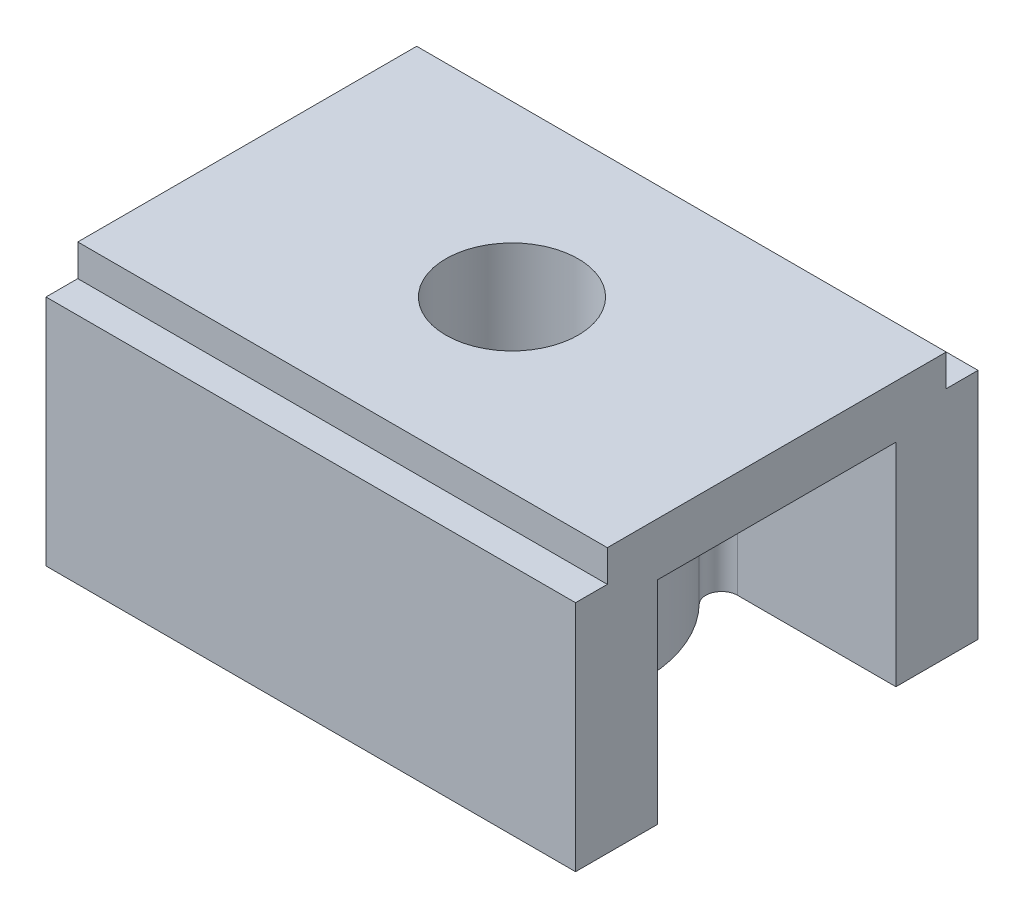
SolidWorks part; units mm, degrees
material "Plain Carbon Steel"
ref_plane "Front Plane" through (0, 0, 0) normal (0, 0, 1) x (1, 0, 0)
ref_plane "Top Plane" through (0, 0, 0) normal (0, 1, 0) x (1, 0, 0)
ref_plane "Right Plane" through (0, 0, 0) normal (1, 0, 0) x (0, 0, -1)
sketch "Channel Profile Sketch" plane through (0, 0, 0) normal (0, 1, 0) x (1, 0, 0)
  line L0 (-50, 22.5) -> (-20.0935, 22.5)
  line L1 (-50, 38) -> (50, 38)
  line L2 (-50, 38) -> (-50, 22.5)
  line L3 (-50, -38) -> (50, -38)
  line L4 (50, 38) -> (50, 22.5)
  line L5 (-50, 38) -> (50, -38) construction
  line L6 (-50, -38) -> (50, 38) construction
  line L7 (-50, -22.5) -> (-20.0935, -22.5)
  line L8 (20.0935, 22.5) -> (50, 22.5)
  line L9 (20.0935, -22.5) -> (50, -22.5)
  line L10 (-50, -22.5) -> (-50, -38)
  line L11 (50, -22.5) -> (50, -38)
  arc A0 (-17.9407, 17.4107) -> (-17.9407, -17.4107) centre (0, 0) ccw
  arc A1 (-17.9407, 17.4107) -> (-20.0935, 22.5) centre (-20.0935, 19.5) ccw
  arc A2 (20.0935, 22.5) -> (17.9407, 17.4107) centre (20.0935, 19.5) ccw
  arc A3 (17.9407, -17.4107) -> (20.0935, -22.5) centre (20.0935, -19.5) ccw
  arc A4 (-20.0935, -22.5) -> (-17.9407, -17.4107) centre (-20.0935, -19.5) ccw
  arc A5 (17.9407, -17.4107) -> (17.9407, 17.4107) centre (0, 0) ccw
  point P0 (0, 0)
  dimension "D5" = 50
  dimension "D6" = 6
  dimension "D7" = 6
  dimension "D8" = 6
  dimension "D9" = 6
  dimension "D1" = 100
  dimension "D2" = 76
  dimension "D3" = 45
  dimension "D4" = 22.5
extrude "Channel Body" add sketch "Channel Profile Sketch" along normal blind 40 contours L3 L11 L9 A3 A5 A2 L8 L4 L1 L2 L0 A1 A0 A4 L7 L10
sketch "Top Plate Sketch" plane through (0, 40, 0) normal (0, 1, 0) x (1, 0, 0)
  line L1 (-50, 38) -> (50, 38)
  line L2 (-50, 38) -> (-50, -38)
  line L3 (-50, -38) -> (50, -38)
  line L4 (50, 38) -> (50, -38)
  line L5 (-50, 38) -> (50, -38) construction
  line L6 (-50, -38) -> (50, 38) construction
  point P0 (0, 0)
extrude "Top Plate" add sketch "Top Plate Sketch" along normal blind 10
sketch "Guide Grooves Sketch" plane through (0, 50, 0) normal (0, 1, 0) x (1, 0, 0)
  line L0 (-50, 32) -> (50, 32)
  line L1 (-50, -32) -> (50, -32)
  line L2 (-50, -38) -> (50, -38) construction
  line L3 (50, 38) -> (-50, 38) construction
  line L4 (50, -38) -> (50, 38) construction
  line L5 (-50, 38) -> (-50, -38) construction
  line L6 (-50, -38) -> (50, -38)
  line L7 (50, -38) -> (50, -32)
  line L8 (50, 38) -> (-50, 38)
  line L9 (-50, 38) -> (-50, 32)
  line L10 (-50, -32) -> (-50, -38)
  line L11 (50, 32) -> (50, 38)
  dimension "D1" = 6
  dimension "D2" = 6
sketch "Bore Sketch" plane through (0, 50, 0) normal (0, 1, 0) x (1, 0, 0)
  circle A0 centre (0, 0) radius 12.5
  dimension "D1" = 25
extrude "Bore Ø25" cut sketch "Bore Sketch" against normal blind 56
extrude "Guide Grooves 6x6" cut sketch "Guide Grooves Sketch" against normal blind 6 contours L1 L7 L6 L10
